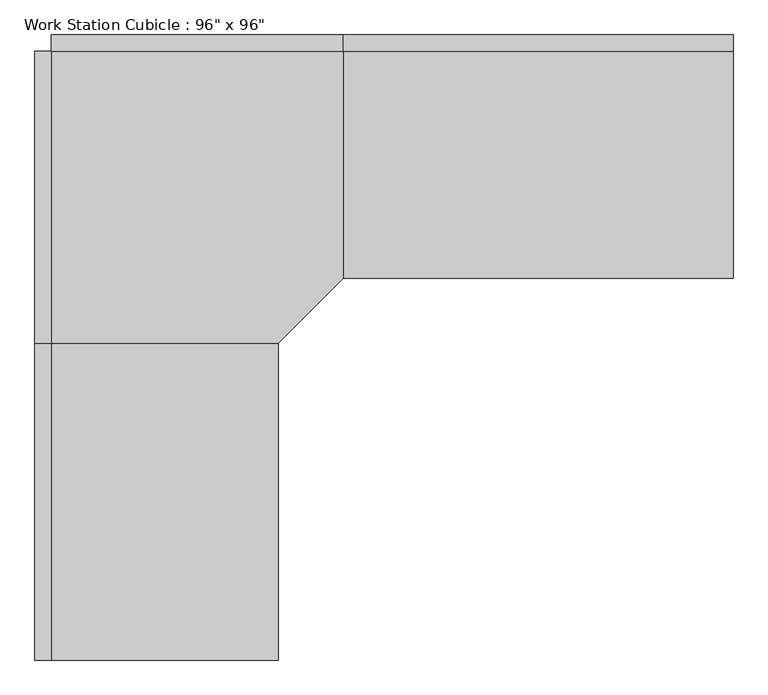
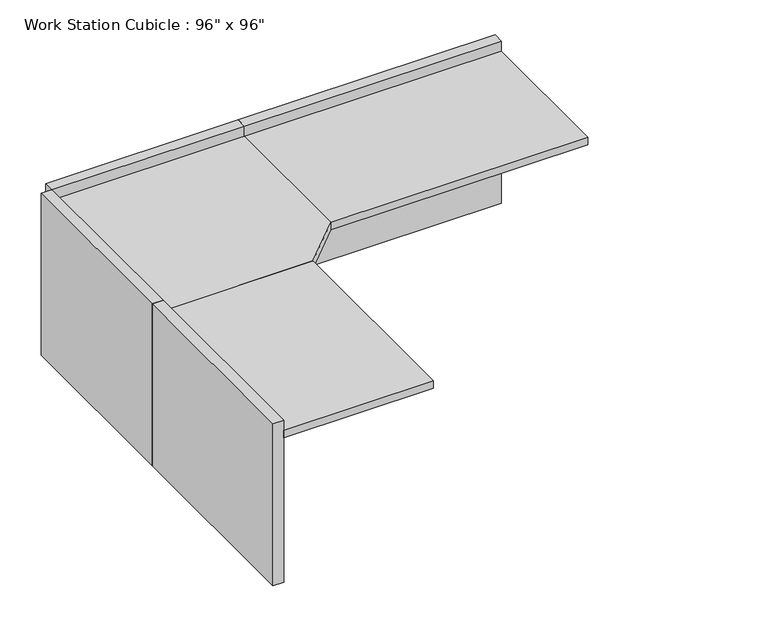
"""IFC4 building model written with IfcOpenShell, lengths in millimetres: furniture geometry."""

from ifc_helpers import new_model, si_unit, frame, origin, origin_with_axes, place, context, project, spatial, polyline, outline, extrude, source, transform, mapped, element, save


def furniture_5916b341(model_context):
    return source(origin(), model_context, "Body", "SweptSolid", [
        extrude(outline(polyline([(-80.9317522, -545.8230076), (833.4682478, -545.8230076), (833.4682478, -1257.0230076), (630.2682478, -1460.2230076), (-80.9317522, -1460.2230076), (-80.9317522, -545.8230076)])), frame((0.0, 0.0, 723.9), z_axis=(0.0, 0.0, 1.0), x_axis=(1.0, 0.0, 0.0)), (0.0, 0.0, 1.0), 38.1),
        extrude(outline(polyline([(630.2682478, -2450.8230076), (-80.9317522, -2450.8230076), (-80.9317522, -1460.2230076), (630.2682478, -1460.2230076), (630.2682478, -2450.8230076)])), frame((0.0, 0.0, 723.9), z_axis=(0.0, 0.0, 1.0), x_axis=(1.0, 0.0, 0.0)), (0.0, 0.0, 1.0), 38.1),
        extrude(outline(polyline([(2052.6682478, -1257.0230076), (833.4682478, -1257.0230076), (833.4682478, -545.8230076), (2052.6682478, -545.8230076), (2052.6682478, -1257.0230076)])), frame((0.0, 0.0, 723.9), z_axis=(0.0, 0.0, 1.0), x_axis=(1.0, 0.0, 0.0)), (0.0, 0.0, 1.0), 38.1),
        extrude(outline(polyline([(2052.6682478, -545.8230076), (833.4682478, -545.8230076), (833.4682478, -495.0230076), (2052.6682478, -495.0230076), (2052.6682478, -545.8230076)])), origin_with_axes(), (0.0, 0.0, 1.0), 812.8),
        extrude(outline(polyline([(833.4682478, -545.8230076), (-80.9317522, -545.8230076), (-80.9317522, -495.0230076), (833.4682478, -495.0230076), (833.4682478, -545.8230076)])), origin_with_axes(), (0.0, 0.0, 1.0), 812.8),
        extrude(outline(polyline([(-80.9317522, -1460.2230076), (-131.7317522, -1460.2230076), (-131.7317522, -545.8230076), (-80.9317522, -545.8230076), (-80.9317522, -1460.2230076)])), origin_with_axes(), (0.0, 0.0, 1.0), 812.8),
        extrude(outline(polyline([(-80.9317522, -2450.8230076), (-131.7317522, -2450.8230076), (-131.7317522, -1460.2230076), (-80.9317522, -1460.2230076), (-80.9317522, -2450.8230076)])), origin_with_axes(), (0.0, 0.0, 1.0), 812.8),
    ])


if __name__ == "__main__":
    model = new_model("IFC4")
    model_context = context("Model", 3, world=origin())
    ifc_project = project(units=[si_unit("LENGTHUNIT", "METRE", prefix="MILLI")], contexts=[model_context])
    site = spatial("IfcSite", under=ifc_project)
    building = spatial("IfcBuilding", under=site)
    placement = place(None, origin())
    furniture_shape = furniture_5916b341(model_context)
    element("IfcFurniture", 1, ObjectType="Work Station Cubicle : 96\" x 96\"", at=placement, inside=building, context=model_context, shape_type="MappedRepresentation", body=[
        mapped(furniture_shape, transform((0.0, 0.0, 0.0), x_axis=(1.0, 0.0, 0.0), y_axis=(0.0, 1.0, 0.0), z_axis=(0.0, 0.0, 1.0))),
    ])
    save(model, "model.ifc")

# Revit data of these elements
# Type "Work Station Cubicle : 96\" x 96\""
#   Assembly Code = "E2020"
#   Desktop Height = 2' - 6"
#   Desktop1 Width = 2' - 4"
#   Desktop2 Width = 2' - 4"
#   Panel Height = 2' - 8"
#   Panel1 Length = 3' - 3"
#   Panel2 Length = 4' - 0"
#   Cube Panel Material = Textile - Light Gray
#   Work Top Material = Laminate, Ivory, Matte
#   Default Elevation = 0
# Element 1 (IfcFurniture, "Work Station Cubicle : 96\" x 96\"")
#   Materials on its faces: "Textile - Light Gray", "Laminate, Ivory, Matte"
# Materials
#   "Textile - Light Gray": class "Fabric", colour RGB 204 204 204, transparency 0
#   "Laminate, Ivory, Matte": class "Plastic", colour RGB 247 247 239, transparency 0, Description = "Plastic Laminate - Ivory, Matte", Cost = 0
